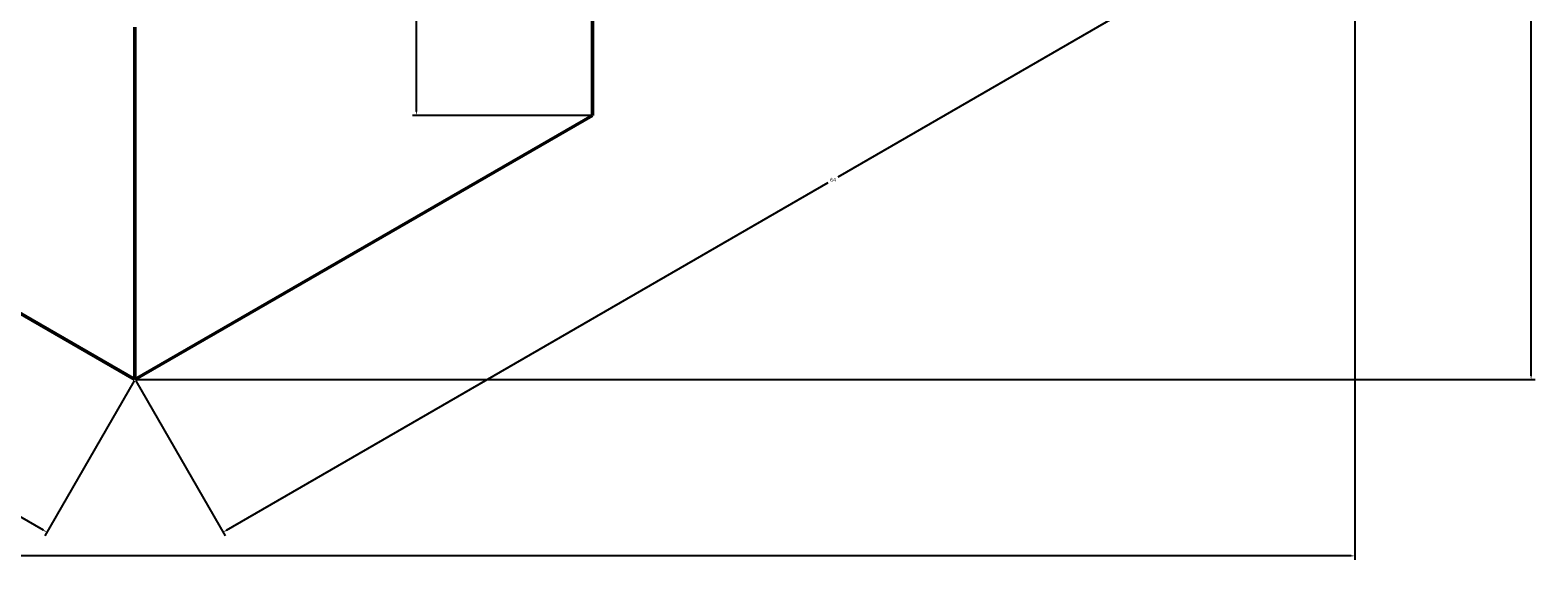
# Model space of a CAD drawing. Units: millimetres. Extents: x 2919 to 3075, y 2801 to 2951.
# Tile 10 of 14: x 3006 to 3075, y 2801 to 2825. Entities that reach past the tile are written whole.
import ezdxf

# ---------------------------------------------------------------- set-up
doc = ezdxf.new("R2010")
doc.units = ezdxf.units.MM
doc.layers.add('M-DIMS', color=2, linetype='Continuous', lineweight=18)
doc.layers.add('M-OUTL', color=7, linetype='Continuous', lineweight=50)
doc.styles.get("Standard").update_dxf_attribs({"font": 'arial.ttf'})
doc.dimstyles.get("Standard").update_dxf_attribs({"dimtxt": 0.18, "dimasz": 0.18, "dimexe": 0.18, "dimexo": 0.0625, "dimgap": 0.09, "dimtad": 0, "dimtih": 1, "dimtoh": 1, "dimdec": 4, "dimzin": 0, "dimdsep": 46, "dimtxsty": 'Standard', "dimcen": 0.09, "dimadec": 0, "dimazin": 0, "dimtfac": 1, "dimtdec": 4, "dimtofl": 0, "dimtmove": 0, "dimatfit": 3, "dimfxl": 1, "dimtolj": 1, "dimtzin": 0, "dimarcsym": 0})

# ---------------------------------------------------------------- blocks, each defined once
blk = doc.blocks.new('*D1')
at = {"layer": 'Defpoints', "color": 0, "transparency": 16777216}
for p in [(2987.323, 2944.203), (3074.337, 2944.203), (3010.912, 2808.893)]:
    blk.add_point(p, dxfattribs=at)
at = {"layer": 'M-DIMS', "color": 0, "lineweight": -2, "transparency": 16777216}
for p, q in [((2987.386, 2944.203), (3074.517, 2944.203)), ((3074.337, 2944.023), (3074.337, 2876.73)), ((3074.337, 2809.073), (3074.337, 2876.366)), ((3010.974, 2808.893), (3074.517, 2808.893))]:
    blk.add_line(p, q, dxfattribs=at)
at = {"layer": 'M-DIMS', "color": 0, "transparency": 16777216}
for points in [[(3074.307, 2944.023), (3074.367, 2944.023), (3074.337, 2944.203)], [(3074.307, 2809.073), (3074.367, 2809.073), (3074.337, 2808.893)]]:
    blk.add_solid(points, dxfattribs=at)
at = {"layer": 'M-DIMS', "color": 0, "transparency": 16777216, "insert": (3074.337, 2876.548), "char_height": 0.18, "attachment_point": 5}
blk.add_mtext('\\A1;135.3', dxfattribs=at)
blk = doc.blocks.new('*D2')
at = {"layer": 'Defpoints', "color": 0, "transparency": 16777216}
for p in [(2927.773, 2856.893), (3066.337, 2840.893), (3066.337, 2800.893)]:
    blk.add_point(p, dxfattribs=at)
at = {"layer": 'M-DIMS', "color": 0, "lineweight": -2, "transparency": 16777216}
for p, q in [((2927.773, 2856.831), (2927.773, 2800.713)), ((3066.337, 2840.831), (3066.337, 2800.713)), ((2927.953, 2800.893), (2996.6, 2800.893)), ((3066.157, 2800.893), (2997.51, 2800.893))]:
    blk.add_line(p, q, dxfattribs=at)
at = {"layer": 'M-DIMS', "color": 0, "transparency": 16777216}
for points in [[(2927.953, 2800.923), (2927.953, 2800.863), (2927.773, 2800.893)], [(3066.157, 2800.923), (3066.157, 2800.863), (3066.337, 2800.893)]]:
    blk.add_solid(points, dxfattribs=at)
at = {"layer": 'M-DIMS', "color": 0, "transparency": 16777216, "insert": (2997.055, 2800.893), "char_height": 0.18, "attachment_point": 5}
blk.add_mtext('\\A1;138.56', dxfattribs=at)
blk = doc.blocks.new('*D3')
at = {"layer": 'Defpoints', "color": 0, "transparency": 16777216}
for p in [(2927.773, 2856.893), (2923.773, 2849.965), (3010.912, 2808.893)]:
    blk.add_point(p, dxfattribs=at)
at = {"layer": 'M-DIMS', "color": 0, "lineweight": -2, "transparency": 16777216}
for p, q in [((2927.742, 2856.839), (2923.683, 2849.809)), ((2923.929, 2849.875), (2965.124, 2826.091)), ((3006.756, 2802.055), (2965.561, 2825.839)), ((3010.88, 2808.839), (3006.822, 2801.809))]:
    blk.add_line(p, q, dxfattribs=at)
at = {"layer": 'M-DIMS', "color": 0, "transparency": 16777216}
for points in [[(2923.944, 2849.901), (2923.914, 2849.849), (2923.773, 2849.965)], [(3006.771, 2802.081), (3006.741, 2802.029), (3006.912, 2801.965)]]:
    blk.add_solid(points, dxfattribs=at)
at = {"layer": 'M-DIMS', "color": 0, "transparency": 16777216, "insert": (2965.342, 2825.965), "char_height": 0.18, "attachment_point": 5}
blk.add_mtext('\\A1;96', dxfattribs=at)
blk = doc.blocks.new('*D4')
at = {"layer": 'Defpoints', "color": 0, "transparency": 16777216}
for p in [(3066.337, 2840.893), (3010.912, 2808.893), (3014.912, 2801.965)]:
    blk.add_point(p, dxfattribs=at)
at = {"layer": 'M-DIMS', "color": 0, "lineweight": -2, "transparency": 16777216}
for p, q in [((3066.368, 2840.839), (3070.427, 2833.809)), ((3070.181, 2833.875), (3042.843, 2818.092)), ((3015.068, 2802.055), (3042.405, 2817.839)), ((3010.943, 2808.839), (3015.002, 2801.809))]:
    blk.add_line(p, q, dxfattribs=at)
at = {"layer": 'M-DIMS', "color": 0, "transparency": 16777216}
for points in [[(3070.166, 2833.901), (3070.196, 2833.849), (3070.337, 2833.965)], [(3015.053, 2802.081), (3015.083, 2802.029), (3014.912, 2801.965)]]:
    blk.add_solid(points, dxfattribs=at)
at = {"layer": 'M-DIMS', "color": 0, "transparency": 16777216, "insert": (3042.624, 2817.965), "char_height": 0.18, "attachment_point": 5}
blk.add_mtext('\\A1;64', dxfattribs=at)
blk = doc.blocks.new('*D5')
at = {"layer": 'Defpoints', "color": 0, "transparency": 16777216}
for p in [(3023.696, 2836.893), (3031.696, 2836.893), (3031.696, 2820.893)]:
    blk.add_point(p, dxfattribs=at)
at = {"layer": 'M-DIMS', "color": 0, "lineweight": -2, "transparency": 16777216}
for p, q in [((3031.634, 2836.893), (3023.516, 2836.893)), ((3023.696, 2836.713), (3023.696, 2829.075)), ((3023.696, 2821.073), (3023.696, 2828.711)), ((3031.634, 2820.893), (3023.516, 2820.893))]:
    blk.add_line(p, q, dxfattribs=at)
at = {"layer": 'M-DIMS', "color": 0, "transparency": 16777216}
for points in [[(3023.666, 2836.713), (3023.726, 2836.713), (3023.696, 2836.893)], [(3023.666, 2821.073), (3023.726, 2821.073), (3023.696, 2820.893)]]:
    blk.add_solid(points, dxfattribs=at)
at = {"layer": 'M-DIMS', "color": 0, "transparency": 16777216, "insert": (3023.696, 2828.893), "char_height": 0.18, "attachment_point": 5}
blk.add_mtext('\\A1;16', dxfattribs=at)

msp = doc.modelspace()

# ---------------------------------------------------------------- linework, layer by layer
at = {"layer": 'M-OUTL'}
for p, q in [((2927.7732, 2856.8932), (3010.9116, 2808.8932)), ((3031.6962, 2820.8932), (3031.6962, 2836.8932)), ((3010.9116, 2824.8932), (3010.9116, 2808.8932)), ((3010.9116, 2808.8932), (3031.6962, 2820.8932)), ((3010.9116, 2808.8932), (3031.6962, 2820.8932))]:
    msp.add_line(p, q, dxfattribs=at)

# ---------------------------------------------------------------- dimensions: what is measured, and where the dimension line sits
at = {"layer": 'M-DIMS'}
for base, p1, p2, angle, override, picture, middle in [((3074.3372, 2944.2026), (3010.9116, 2808.8932), (2987.3232, 2944.2026), 90, {"dimdec": 1, "dimlfac": 1, "dimrnd": 0, "dimzin": 0, "dimdsep": 46, "dimlunit": 2}, '*D1', (3074.3372, 2876.5479)), ((2923.7732, 2849.965), (3010.9116, 2808.8932), (2927.7732, 2856.8932), 150, {"dimdec": 0, "dimlfac": 1, "dimrnd": 0, "dimzin": 0, "dimdsep": 46, "dimlunit": 2}, '*D3', (2965.3424, 2825.965)), ((3014.9116, 2801.965), (3066.3372, 2840.8932), (3010.9116, 2808.8932), 210, {"dimdec": 0, "dimlfac": 1, "dimrnd": 0, "dimzin": 0, "dimdsep": 46, "dimlunit": 2}, '*D4', (3042.6244, 2817.965)), ((3023.6962, 2836.8932), (3031.6962, 2820.8932), (3031.6962, 2836.8932), 90, {"dimdec": 0, "dimlfac": 1, "dimrnd": 0, "dimzin": 0, "dimdsep": 46, "dimlunit": 2}, '*D5', (3023.6962, 2828.8932))]:
    dim = msp.add_linear_dim(base=base, p1=p1, p2=p2, angle=angle, dimstyle='Standard', override=override, dxfattribs=at)
    dim.commit()
    dim.dimension.update_dxf_attribs({"geometry": picture, "text_midpoint": middle})
dim = msp.add_linear_dim(base=(3066.3372, 2800.8932), p1=(2927.7732, 2856.8932), p2=(3066.3372, 2840.8932), dimstyle='Standard', override={"dimdec": 2, "dimlfac": 1, "dimrnd": 0, "dimzin": 0, "dimdsep": 46, "dimlunit": 2}, dxfattribs=at)
dim.commit()
dim.dimension.update_dxf_attribs({"geometry": '*D2', "text_midpoint": (2997.0552, 2800.8932)})

doc.saveas('drawing.dxf')
